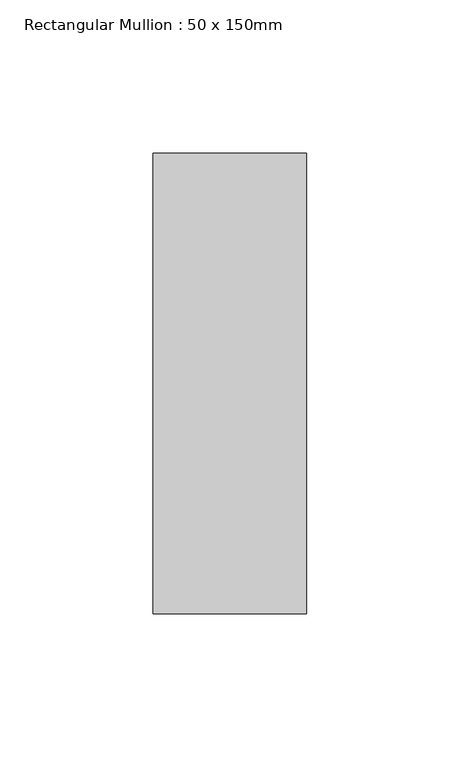
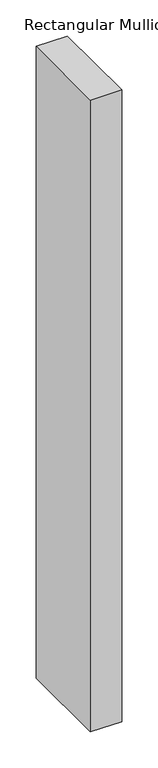
"""IFC4 building model written with IfcOpenShell, lengths in millimetres: member geometry, Rectangular Mullion : 50 x 150mm."""

from ifc_helpers import new_model, si_unit, frame, origin, place, context, project, spatial, polyline, outline, extrude, source, transform, mapped, element, save


def rectangular_mullion_50_x_150mm_561fbe3c(model_context):
    return source(origin(), model_context, "Body", "SweptSolid", [
        extrude(outline(polyline([(0.0, 75.0), (0.0, -75.0), (-50.0, -75.0), (-50.0, 75.0), (0.0, 75.0)])), frame((0.0, 0.0, -1068.0), z_axis=(0.0, 0.0, 1.0), x_axis=(1.0, 0.0, 0.0)), (0.0, 0.0, 1.0), 1068.0),
    ])


if __name__ == "__main__":
    model = new_model("IFC4")
    model_context = context("Model", 3, world=origin())
    ifc_project = project(units=[si_unit("LENGTHUNIT", "METRE", prefix="MILLI")], contexts=[model_context])
    site = spatial("IfcSite", under=ifc_project)
    building = spatial("IfcBuilding", under=site)
    placement = place(None, origin())
    rectangular_mullion_50_x_150mm_shape = rectangular_mullion_50_x_150mm_561fbe3c(model_context)
    element("IfcMember", 1, ObjectType="Rectangular Mullion : 50 x 150mm", at=placement, inside=building, context=model_context, shape_type="MappedRepresentation", body=[
        mapped(rectangular_mullion_50_x_150mm_shape, transform((0.0, 0.0, 0.0), x_axis=(1.0, 0.0, 0.0), y_axis=(0.0, 1.0, 0.0), z_axis=(0.0, 0.0, 1.0))),
    ])
    save(model, "model.ifc")

# Revit data of these elements
# Type "Rectangular Mullion : 50 x 150mm"
#   built-in parameter 1007304 = 0.492126 (stored number, unit not read)
#   built-in parameter 1007301 = 0.082021 (stored number, unit not read)
#   built-in parameter 1007300 = 0.082021 (stored number, unit not read)
# Element 1 (IfcMember, "Rectangular Mullion : 50 x 150mm")
#   Materials on its faces: "Aluminium"
# Materials
#   "Aluminium": class "Metal", colour RGB 247 247 247, transparency 0, Description = "Aluminium 6061", Cost = 0
